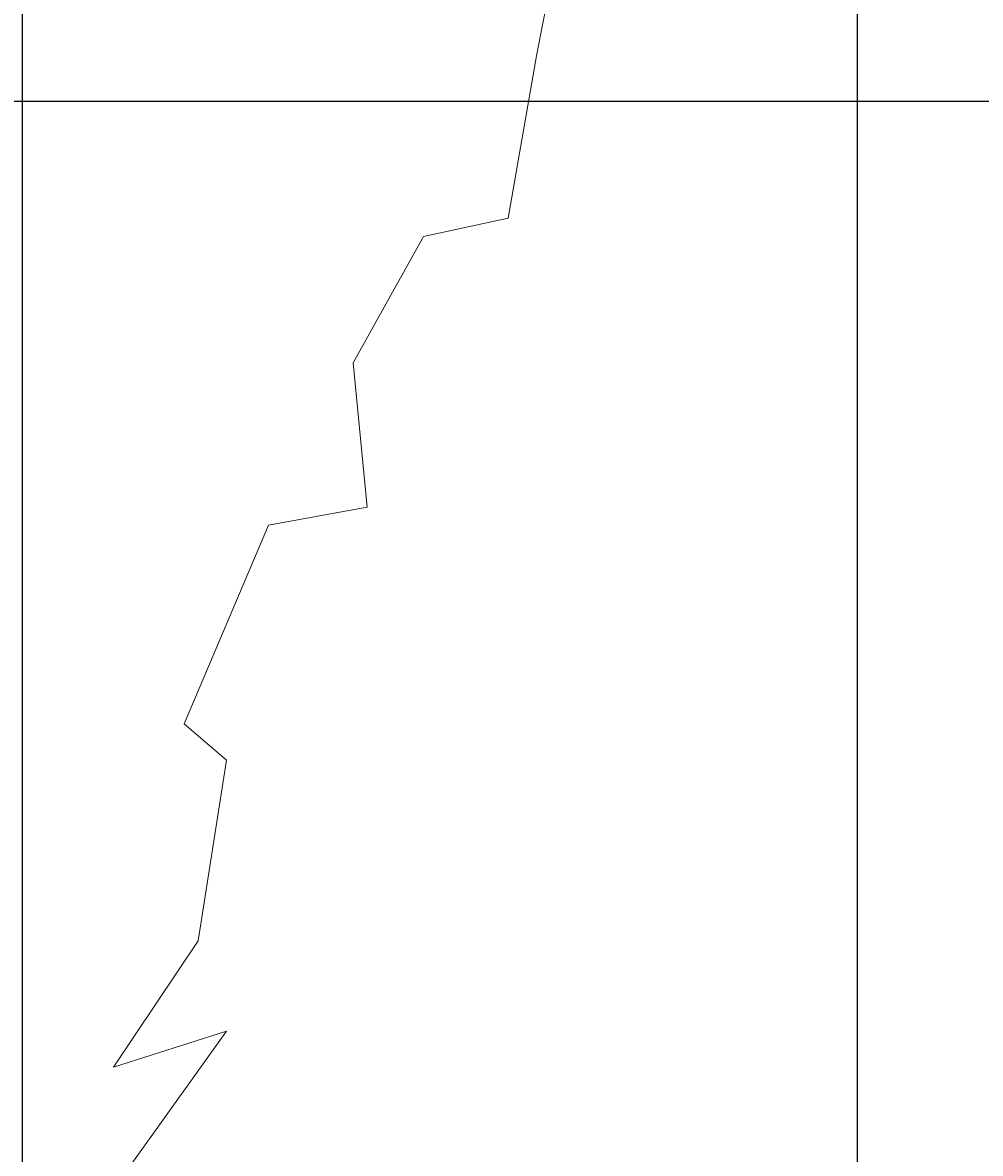
# Model space of a CAD drawing. Units: inches. Extents: x -26 to 776, y -22 to 650.
# Tile 56 of 62: x 426 to 506, y 226 to 321. Entities that reach past the tile are written whole.
import ezdxf

# ---------------------------------------------------------------- set-up
doc = ezdxf.new("R2010")
doc.units = ezdxf.units.IN
doc.header["$MEASUREMENT"] = 0
doc.layers.add('A-ANNO-DIMS', color=2, linetype='Continuous', lineweight=18)
doc.layers.add('L-PLNT-TREE', color=94, linetype='Continuous', lineweight=18)
doc.styles.get("Standard").update_dxf_attribs({"font": 'arial.ttf'})
doc.dimstyles.get("Standard").update_dxf_attribs({"dimtxt": 0.5625, "dimasz": 0.18, "dimexe": 0.18, "dimexo": 0.0625, "dimgap": 0.09, "dimtad": 0, "dimtih": 1, "dimtoh": 1, "dimdec": 4, "dimzin": 0, "dimdsep": 46, "dimlunit": 4, "dimtxsty": 'Standard', "dimcen": 0.09, "dimadec": 0, "dimazin": 0, "dimtfac": 1, "dimtdec": 4, "dimtofl": 0, "dimtmove": 0, "dimatfit": 3, "dimfxl": 1, "dimtolj": 1, "dimtzin": 0, "dimarcsym": 0})

# ---------------------------------------------------------------- blocks, each defined once
blk = doc.blocks.new('Tree - type 2 deciduous elevation')
blk.add_lwpolyline([(-21.158, 150.41), (-21.733, 147.461), (-22.884, 140.825), (-26.334, 140.087), (-29.21, 134.926), (-28.635, 129.028), (-32.661, 128.291), (-36.111, 120.18), (-34.386, 118.706), (-35.536, 111.333), (-38.987, 106.171), (-34.386, 107.646), (-40.712, 98.798)])
blk = doc.blocks.new('*D20')
at = {"layer": 'A-ANNO-DIMS', "color": 0, "lineweight": -2, "transparency": 16777216}
for p, q in [((425.806, 455.472), (775.335, 455.472)), ((775.155, 455.292), (775.155, 235.854)), ((775.155, 15.662), (775.155, 235.1)), ((425.806, 15.482), (775.335, 15.482))]:
    blk.add_line(p, q, dxfattribs=at)
at = {"layer": 'A-ANNO-DIMS', "color": 0, "transparency": 16777216}
for points in [[(775.125, 455.292), (775.185, 455.292), (775.155, 455.472)], [(775.125, 15.662), (775.185, 15.662), (775.155, 15.482)]]:
    blk.add_solid(points, dxfattribs=at)
at = {"layer": 'Defpoints', "color": 0, "transparency": 16777216}
for p in [(425.743, 455.472), (775.155, 455.472), (425.743, 15.482)]:
    blk.add_point(p, dxfattribs=at)
at = {"layer": 'A-ANNO-DIMS', "color": 0, "transparency": 16777216, "insert": (775.155, 235.477), "char_height": 0.5625, "attachment_point": 5}
blk.add_mtext('\\A1;440', dxfattribs=at)
blk = doc.blocks.new('*D28')
at = {"layer": 'A-ANNO-DIMS', "color": 0, "lineweight": -2, "transparency": 16777216}
for p, q in [((285.08, 314.119), (775.335, 314.119)), ((775.155, 313.939), (775.155, 243.141)), ((775.155, 171.597), (775.155, 242.396)), ((285.08, 171.417), (775.335, 171.417))]:
    blk.add_line(p, q, dxfattribs=at)
at = {"layer": 'A-ANNO-DIMS', "color": 0, "transparency": 16777216}
for points in [[(775.125, 313.939), (775.185, 313.939), (775.155, 314.119)], [(775.125, 171.597), (775.185, 171.597), (775.155, 171.417)]]:
    blk.add_solid(points, dxfattribs=at)
at = {"layer": 'Defpoints', "color": 0, "transparency": 16777216}
for p in [(285.018, 314.119), (775.155, 314.119), (285.018, 171.417)]:
    blk.add_point(p, dxfattribs=at)
at = {"layer": 'A-ANNO-DIMS', "color": 0, "transparency": 16777216, "insert": (775.155, 242.768), "char_height": 0.5625, "attachment_point": 5}
blk.add_mtext('\\A1;142.7', dxfattribs=at)
blk = doc.blocks.new('*D39')
at = {"layer": 'A-ANNO-DIMS', "color": 0, "lineweight": -2, "transparency": 16777216}
for p, q in [((289.242, 15.545), (289.242, 649.856)), ((289.422, 649.676), (356.478, 649.676)), ((425.563, 649.676), (358.508, 649.676)), ((425.743, 15.545), (425.743, 649.856))]:
    blk.add_line(p, q, dxfattribs=at)
at = {"layer": 'A-ANNO-DIMS', "color": 0, "transparency": 16777216}
for points in [[(289.422, 649.706), (289.422, 649.646), (289.242, 649.676)], [(425.563, 649.706), (425.563, 649.646), (425.743, 649.676)]]:
    blk.add_solid(points, dxfattribs=at)
at = {"layer": 'Defpoints', "color": 0, "transparency": 16777216}
for p in [(425.743, 649.676), (289.242, 15.482), (425.743, 15.482)]:
    blk.add_point(p, dxfattribs=at)
at = {"layer": 'A-ANNO-DIMS', "color": 0, "transparency": 16777216, "insert": (357.493, 649.676), "char_height": 0.5625, "attachment_point": 5}
blk.add_mtext('\\A1;136.5', dxfattribs=at)
blk = doc.blocks.new('*D40')
at = {"layer": 'A-ANNO-DIMS', "color": 0, "lineweight": -2, "transparency": 16777216}
for p, q in [((425.743, 15.545), (425.743, 649.856)), ((425.923, 649.676), (459.646, 649.676)), ((495.451, 649.676), (461.728, 649.676)), ((495.631, 15.545), (495.631, 649.856))]:
    blk.add_line(p, q, dxfattribs=at)
at = {"layer": 'A-ANNO-DIMS', "color": 0, "transparency": 16777216}
for points in [[(425.923, 649.706), (425.923, 649.646), (425.743, 649.676)], [(495.451, 649.706), (495.451, 649.646), (495.631, 649.676)]]:
    blk.add_solid(points, dxfattribs=at)
at = {"layer": 'Defpoints', "color": 0, "transparency": 16777216}
for p in [(495.631, 649.676), (425.743, 15.482), (495.631, 15.482)]:
    blk.add_point(p, dxfattribs=at)
at = {"layer": 'A-ANNO-DIMS', "color": 0, "transparency": 16777216, "insert": (460.687, 649.676), "char_height": 0.5625, "attachment_point": 5}
blk.add_mtext('\\A1;69.89', dxfattribs=at)

msp = doc.modelspace()

# ---------------------------------------------------------------- block references
at = {"layer": 'L-PLNT-TREE', "xscale": 2.050905272406618, "yscale": 2.050905272406618, "zscale": 2.050905272406618}
msp.add_blockref('Tree - type 2 deciduous elevation', (513.3241, 15.4824), dxfattribs=at)

# ---------------------------------------------------------------- dimensions: what is measured, and where the dimension line sits
at = {"layer": 'A-ANNO-DIMS'}
for base, p1, p2, override, picture, middle in [((425.7434, 649.6763), (289.2424, 15.4824), (425.7434, 15.4824), {"dimdec": 1, "dimlfac": 1, "dimrnd": 0, "dimzin": 0, "dimdsep": 46, "dimlunit": 2}, '*D39', (357.4929, 649.6763)), ((495.6309, 649.6763), (425.7434, 15.4824), (495.6309, 15.4824), {"dimdec": 2, "dimlfac": 1, "dimrnd": 0, "dimzin": 0, "dimdsep": 46, "dimlunit": 2}, '*D40', (460.6872, 649.6763))]:
    dim = msp.add_linear_dim(base=base, p1=p1, p2=p2, dimstyle='Standard', override=override, dxfattribs=at)
    dim.commit()
    dim.dimension.update_dxf_attribs({"geometry": picture, "text_midpoint": middle})
for base, p1, p2, override, picture, middle in [((775.1553, 455.4717), (425.7434, 15.4824), (425.7434, 455.4717), {"dimdec": 0, "dimlfac": 1, "dimrnd": 0, "dimzin": 0, "dimdsep": 46, "dimlunit": 2}, '*D20', (775.1553, 235.477)), ((775.1553, 314.119), (285.0179, 171.4173), (285.0179, 314.119), {"dimdec": 1, "dimlfac": 1, "dimrnd": 0, "dimzin": 0, "dimdsep": 46, "dimlunit": 2}, '*D28', (775.1553, 242.7682))]:
    dim = msp.add_linear_dim(base=base, p1=p1, p2=p2, angle=90, dimstyle='Standard', override=override, dxfattribs=at)
    dim.commit()
    dim.dimension.update_dxf_attribs({"geometry": picture, "text_midpoint": middle})

doc.saveas('drawing.dxf')
